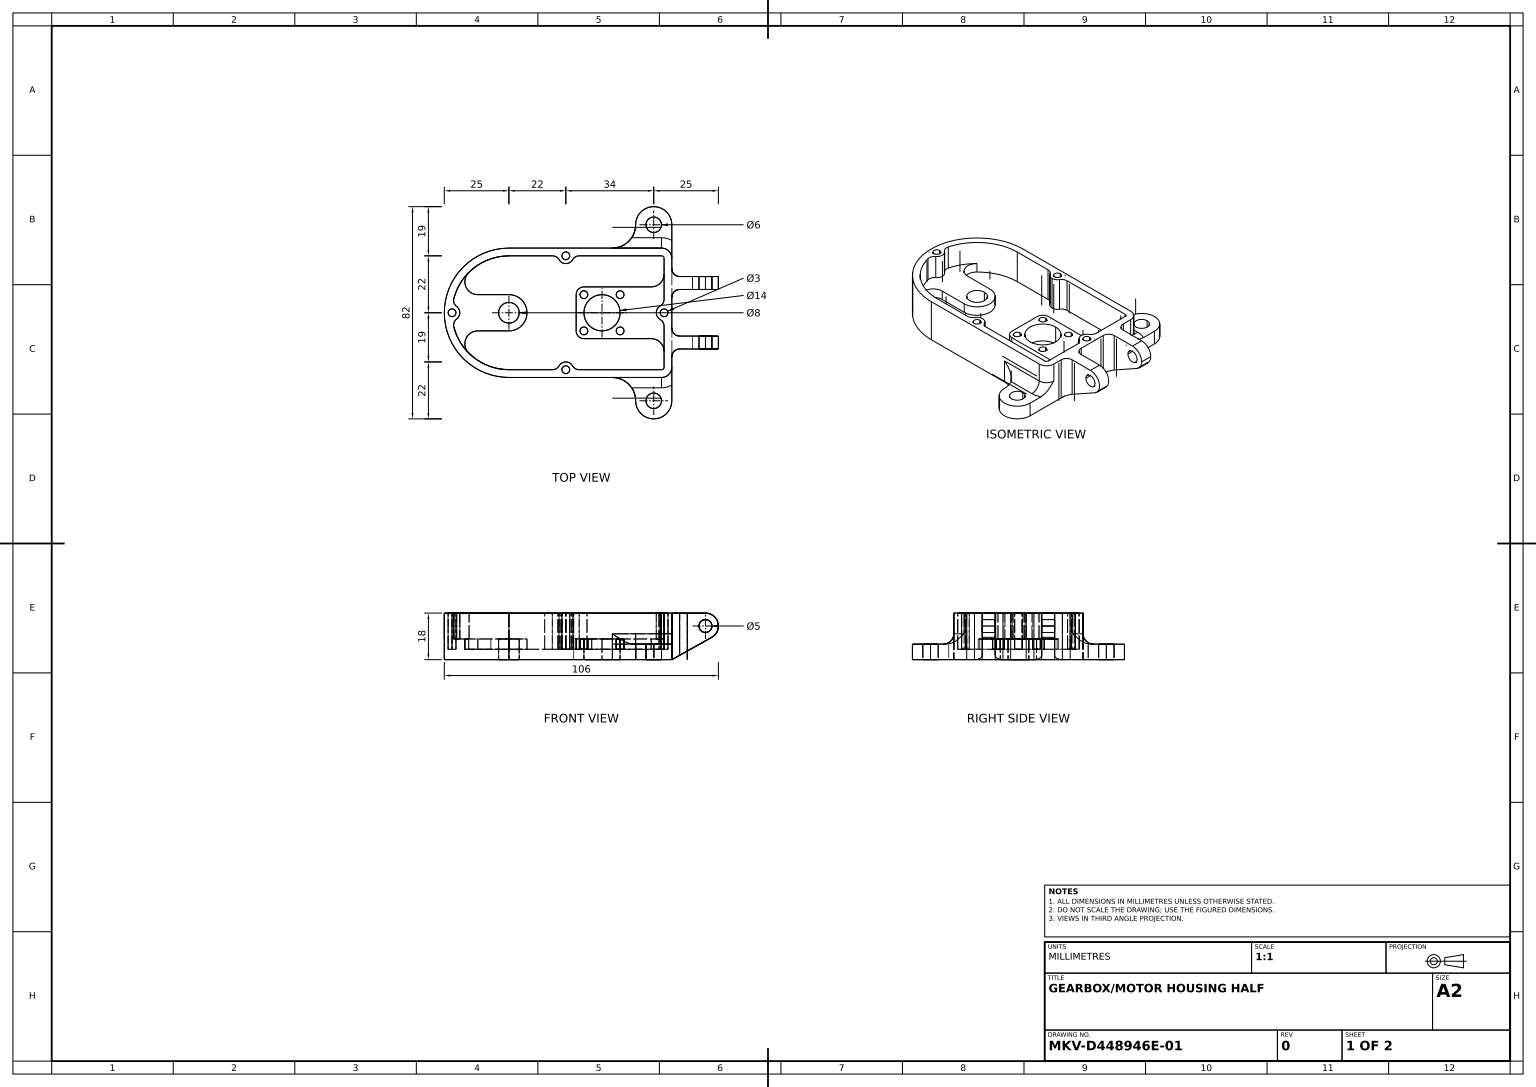
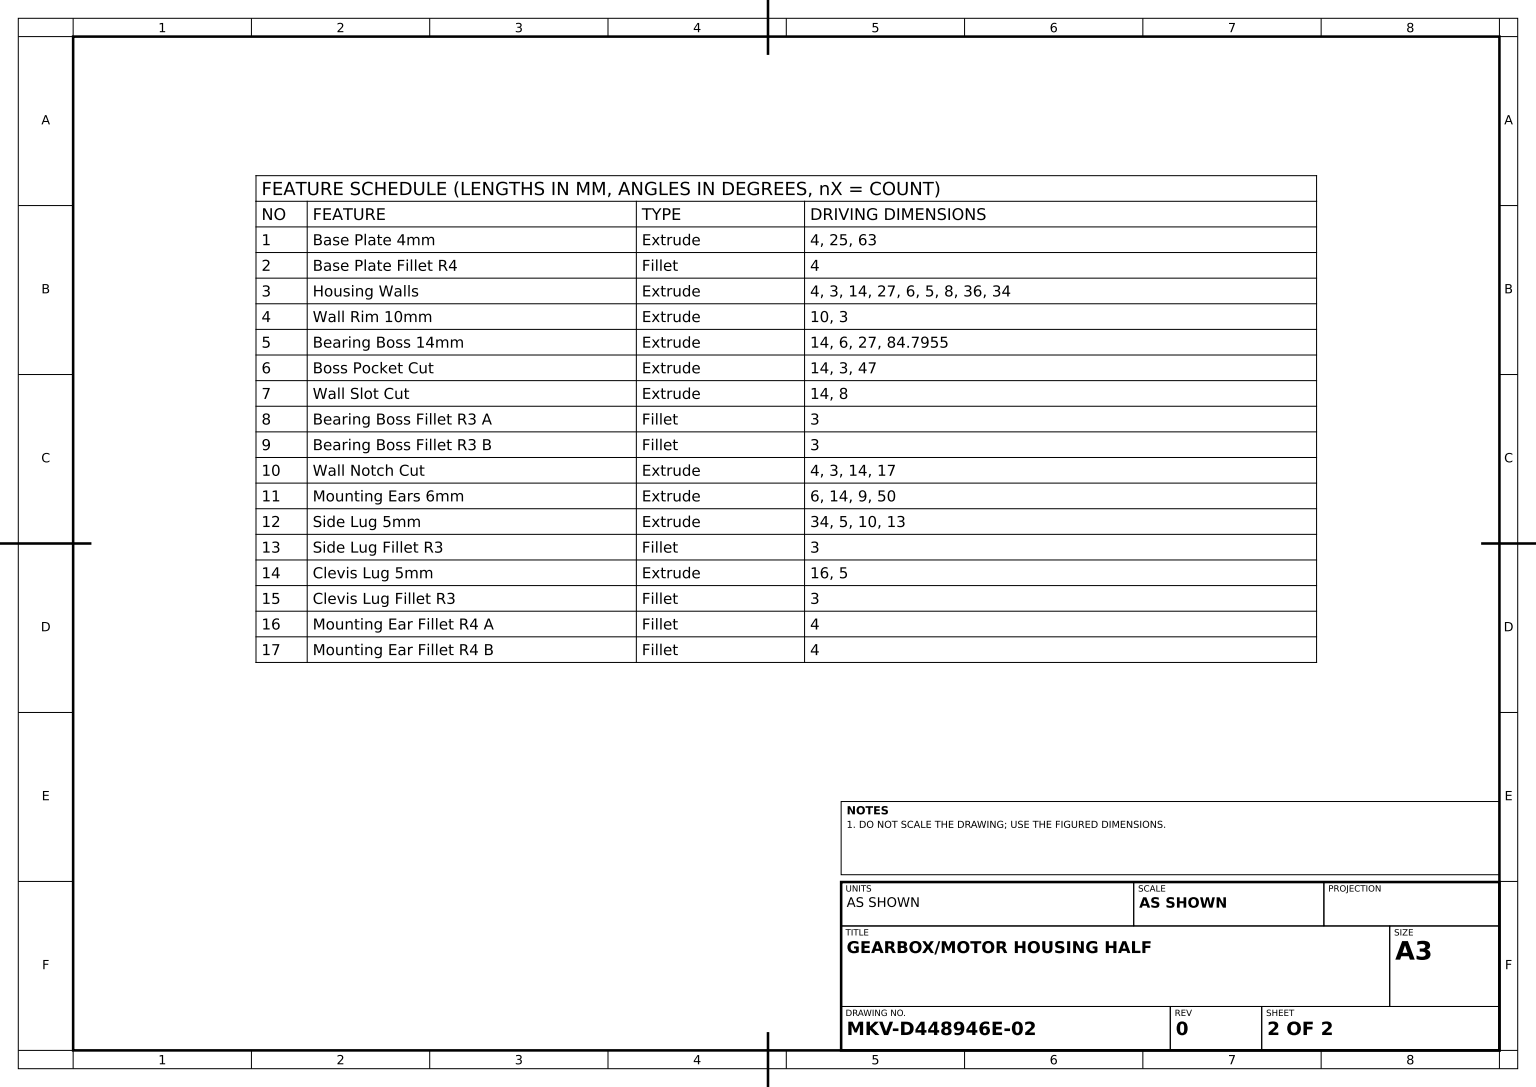
SolidWorks part; units mm, degrees
material "Plain Carbon Steel"
ref_plane "Front Plane" through (0, 0, 0) normal (0, 0, 1) x (1, 0, 0)
ref_plane "Top Plane" through (0, 0, 0) normal (0, 1, 0) x (1, 0, 0)
ref_plane "Right Plane" through (0, 0, 0) normal (1, 0, 0) x (0, 0, -1)
sketch "Base Plate Sketch" plane through (0, 0, 0) normal (0, 1, 0) x (1, 0, 0)
  line L0 (0, 0) -> (-63, 0)
  line L2 (-63, 50) -> (0, 50)
  line L3 (0, 50) -> (0, 0)
  arc A0 (-63, 50) -> (-63, 0) centre (-63, 25) ccw
  dimension "D1" = 25
  dimension "D2" = 63
extrude "Base Plate 4mm" add sketch "Base Plate Sketch" along normal blind 4
fillet "Base Plate Fillet R4" radius 4 2 edges at (0, 2, -50) (0, 2, 0)
sketch "Housing Wall Sketch" plane through (0, 4, 0) normal (0, 1, 0) x (1, 0, 0)
  line L0 (-63, 50) -> (-4, 50)
  line L1 (0, 46) -> (0, 4)
  line L2 (0, 4) -> (0, 46) construction
  line L3 (-63, 0) -> (-4, 0)
  line L4 (-63, 3) -> (-4, 3)
  line L5 (-3, 46) -> (-3, 4)
  line L6 (-63, 47) -> (-4, 47)
  line L8 (-63, 32) -> (-75.0416, 32)
  line L9 (-63, 18) -> (-75.0416, 18)
  line L10 (-37, 32) -> (-37, 18)
  line L17 (-34, 35) -> (-8, 35)
  line L18 (-34, 15) -> (-8, 15)
  arc A0 (-4, 50) -> (0, 46) centre (-4, 46) cw
  arc A1 (-4, 0) -> (0, 4) centre (-4, 4) ccw construction
  arc A2 (-63, 50) -> (-63, 0) centre (-63, 25) ccw
  arc A3 (-4, 0) -> (0, 4) centre (-4, 4) ccw
  arc A4 (-63, 47) -> (-63, 3) centre (-63, 25) ccw
  arc A5 (-4, 3) -> (-3, 4) centre (-4, 4) ccw
  arc A6 (-4, 47) -> (-3, 46) centre (-4, 46) cw
  circle A7 centre (-27, 25) radius 7
  arc A11 (-37, 18) -> (-34, 15) centre (-34, 18) ccw
  arc A12 (-34, 35) -> (-37, 32) centre (-34, 32) ccw
  arc A13 (-3, 40) -> (-8, 35) centre (-8, 40) cw
  arc A14 (-8, 15) -> (-3, 10) centre (-8, 10) cw
  circle A15 centre (-63, 25) radius 7
  circle A16 centre (-63, 25) radius 4
  arc A17 (-78.5832, 40.5294) -> (-75.0416, 32) centre (-75.0416, 37) ccw
  arc A18 (-75.0416, 18) -> (-78.5832, 9.4706) centre (-75.0416, 13) ccw
  point P32 (-88, 15)
  point P33 (-3, 15)
  point P34 (-88, 35)
  point P35 (-3, 35)
  point P36 (0, 25)
  line M7 (0, 4) -> (0, 46)
  arc M8 (0, 46) -> (-4, 50) centre (-4, 46) ccw
  line M9 (-4, 50) -> (-63, 50)
  arc M10 (-63, 50) -> (-63, 0) centre (-63, 25) ccw
  line M11 (-63, 0) -> (-4, 0)
  arc M12 (-4, 0) -> (0, 4) centre (-4, 4) ccw
  dimension "D1" = 3
  dimension "D2" = 14
  dimension "D6" = 5
  dimension "D7" = 36
  dimension "D8" = 5
  dimension "D9" = 6
  dimension "D10" = 5
  dimension "D11" = 5
  dimension "D3" = 14
  dimension "D4" = 8
  dimension "D5" = 27
  dimension "D12" = 34
extrude "Housing Walls" add sketch "Housing Wall Sketch" along normal blind 4 contours A18 L9 A15 L8 A17 A4 | A15 A16 | L18 A14 L5 A13 L17 A12 L10 A11 A7 | L6 A6 L5 A5 L4 A4 M12 M7 M8 M9 M10 M11
sketch "Wall Rim Sketch" plane through (0, 8, 0) normal (0, 1, 0) x (1, 0, 0)
  line L0 (-63, 50) -> (-4, 50)
  line L1 (-63, 0) -> (-4, 0)
  line L2 (0, 46) -> (0, 4)
  line L3 (-63, 3) -> (-4, 3)
  line L4 (-3, 46) -> (-3, 4)
  line L5 (-63, 47) -> (-4, 47)
  arc A0 (-63, 50) -> (-63, 0) centre (-63, 25) ccw
  arc A1 (-4, 0) -> (0, 4) centre (-4, 4) ccw
  arc A2 (-4, 50) -> (0, 46) centre (-4, 46) cw
  arc A3 (-63, 47) -> (-63, 3) centre (-63, 25) ccw
  arc A4 (-4, 3) -> (-3, 4) centre (-4, 4) ccw
  arc A5 (-4, 47) -> (-3, 46) centre (-4, 46) cw
  dimension "D1" = 3
extrude "Wall Rim 10mm" add sketch "Wall Rim Sketch" along normal blind 10
sketch "Bearing Boss Sketch" plane through (0, 18, 0) normal (0, 1, 0) x (1, 0, 0)
  line L0 (-4, 47) -> (-63, 47) construction
  line L1 (-63, 3) -> (-4, 3) construction
  line L2 (-3, 10) -> (-3, 40) construction
  line L3 (-63, 25) -> (-27, 25)
  line L4 (-44, 47) -> (-38, 47)
  line L5 (-3, 28) -> (-3, 22)
  line L6 (-44, 3) -> (-38, 3)
  line L7 (0, 4) -> (0, 46) construction
  arc A0 (-44, 47) -> (-38, 47) centre (-41, 47) ccw
  arc A3 (-38, 3) -> (-44, 3) centre (-41, 3) ccw
  arc A5 (-3, 28) -> (-3, 22) centre (-3, 25) ccw
  arc A7 (-78.5832, 40.5294) -> (-78.5832, 9.4706) centre (-63, 25) ccw construction
  arc A8 (-84.7955, 22.007) -> (-84.7955, 27.993) centre (-85, 25) ccw
  arc A9 (-84.7955, 27.993) -> (-84.7955, 22.007) centre (-63, 25) ccw
  line M7 (-4, 3) -> (-63, 3)
  arc M8 (-63, 3) -> (-63, 47) centre (-63, 25) cw
  line M9 (-63, 47) -> (-4, 47)
  line M11 (-3, 46) -> (-3, 4)
  dimension "D1" = 6
  dimension "D2" = 27
  dimension "D3" = 84.7955
  dimension "D4" = 6
  dimension "D5" = 14
  dimension "D6" = 14
extrude "Bearing Boss 14mm" add sketch "Bearing Boss Sketch" against normal blind 14 contours A8 M8 | A3 M7 | A5 M11 | A0 M9
sketch "Boss Pocket Sketch" plane through (0, 18, 0) normal (0, 1, 0) x (1, 0, 0)
  line L1 (-4, 50) -> (-63, 50) construction
  circle A0 centre (-85, 25) radius 1.5
  circle A1 centre (-41, 3) radius 1.5
  circle A2 centre (-41, 47) radius 1.5
  circle A3 centre (-3, 25) radius 1.5
  dimension "D1" = 3
  dimension "D2" = 3
  dimension "D3" = 3
  dimension "D4" = 3
  dimension "D5" = 47
extrude "Boss Pocket Cut" cut sketch "Boss Pocket Sketch" against normal blind 14
sketch "Wall Slot Sketch" plane through (0, 4, 0) normal (0, 1, 0) x (1, 0, 0)
  circle A0 centre (-63, 25) radius 4
  circle A1 centre (-27, 25) radius 7
  dimension "D1" = 8
  dimension "D2" = 14
extrude "Wall Slot Cut" cut sketch "Wall Slot Sketch" against normal blind 14
fillet "Bearing Boss Fillet R3 A" radius 3 2 edges at (-84.7955, 13, -22.007) (-84.7955, 13, -27.993)
fillet "Bearing Boss Fillet R3 B" radius 3 6 edges at (-38, 11, -3) (-44, 11, -3) (-3, 13, -28) (-3, 13, -22) (-44, 11, -47) (-38, 11, -47)
sketch "Wall Notch Sketch" plane through (0, 8, 0) normal (0, 1, 0) x (1, 0, 0)
  line L0 (-37, 32) -> (-37, 18) construction
  line L1 (-34, 35) -> (-8, 35) construction
  circle A0 centre (-34, 32) radius 1.5
  circle A1 centre (-20, 32) radius 1.5
  circle A2 centre (-20, 18) radius 1.5
  circle A3 centre (-34, 18) radius 1.5
  point P0 (-27, 25)
  dimension "D1" = 3
  dimension "D2" = 3
  dimension "D3" = 14
  dimension "D4" = 3
  dimension "D5" = 3
  dimension "D6" = 17
extrude "Wall Notch Cut" cut sketch "Wall Notch Sketch" against normal blind 4
sketch "Mounting Ear Sketch" plane through (0, 0, 0) normal (0, -1, 0) x (1, 0, 0)
  line L2 (0, 9) -> (0, -4)
  line L3 (-4, -50) -> (-63, -50) construction
  line L4 (-23, -50) -> (-4, -50)
  line L5 (-23, 0) -> (-4, 0)
  line L6 (0, -46) -> (0, -59)
  arc A0 (0, 9) -> (-14, 9) centre (-7, 9) ccw
  circle A1 centre (-7, 9) radius 3
  circle A2 centre (-7, -59) radius 3
  arc A3 (0, -59) -> (-14, -59) centre (-7, -59) cw
  arc A4 (-23, -50) -> (-14, -59) centre (-23, -59) cw
  arc A5 (-4, -50) -> (0, -46) centre (-4, -46) ccw
  arc A6 (-23, 0) -> (-14, 9) centre (-23, 9) ccw
  arc A7 (-4, 0) -> (0, -4) centre (-4, -4) cw
  dimension "D1" = 14
  dimension "D2" = 6
  dimension "D3" = 9
  dimension "D4" = 50
extrude "Mounting Ears 6mm" add sketch "Mounting Ear Sketch" against normal blind 6
ref_plane "Side Lug Plane 34mm" through (0, 0, -34) normal (0, 0, 1) x (1, 0, 0)
sketch "Side Lug Sketch" plane through (0, 0, -34) normal (0, 0, 1) x (1, 0, 0)
  line L0 (0, 18) -> (13, 18)
  line L1 (0, 0) -> (15.4407, 8.6362)
  line L2 (0, 18) -> (0, 0)
  arc A0 (15.4407, 8.6362) -> (13, 18) centre (13, 13) ccw
  circle A1 centre (13, 13) radius 2.5
  dimension "D1" = 10
  dimension "D2" = 5
  dimension "D3" = 13
  dimension "D4" = 5
extrude "Side Lug 5mm" add sketch "Side Lug Sketch" against normal blind 5
fillet "Side Lug Fillet R3" radius 3 2 edges at (0, 9, -39) (0, 9, -34)
ref_plane "Clevis Lug Plane 16mm" through (0, 0, -16) normal (0, 0, 1) x (1, 0, 0)
sketch "Clevis Lug Sketch" plane through (0, 0, -16) normal (0, 0, 1) x (1, 0, 0)
  line L0 (0, 18) -> (0, 0)
  line L1 (0, 0) -> (15.4407, 8.6362)
  line L2 (0, 18) -> (13, 18)
  line L3 (13, 18) -> (3, 18) construction
  arc A0 (15.4407, 8.6362) -> (13, 18) centre (13, 13) ccw construction
  circle A1 centre (13, 13) radius 2.5
  arc A2 (13, 18) -> (15.4407, 8.6362) centre (13, 13) cw
  dimension "D1" = 5
extrude "Clevis Lug 5mm" add sketch "Clevis Lug Sketch" along normal blind 5
fillet "Clevis Lug Fillet R3" radius 3 2 edges at (0, 9, -16) (0, 9, -11)
fillet "Mounting Ear Fillet R4 A" radius 4 2 edges at (-1.1716, 6, -1.1716) (-13.5, 6, 0)
fillet "Mounting Ear Fillet R4 B" radius 4 2 edges at (-1.1716, 6, -48.8284) (-13.5, 6, -50)
